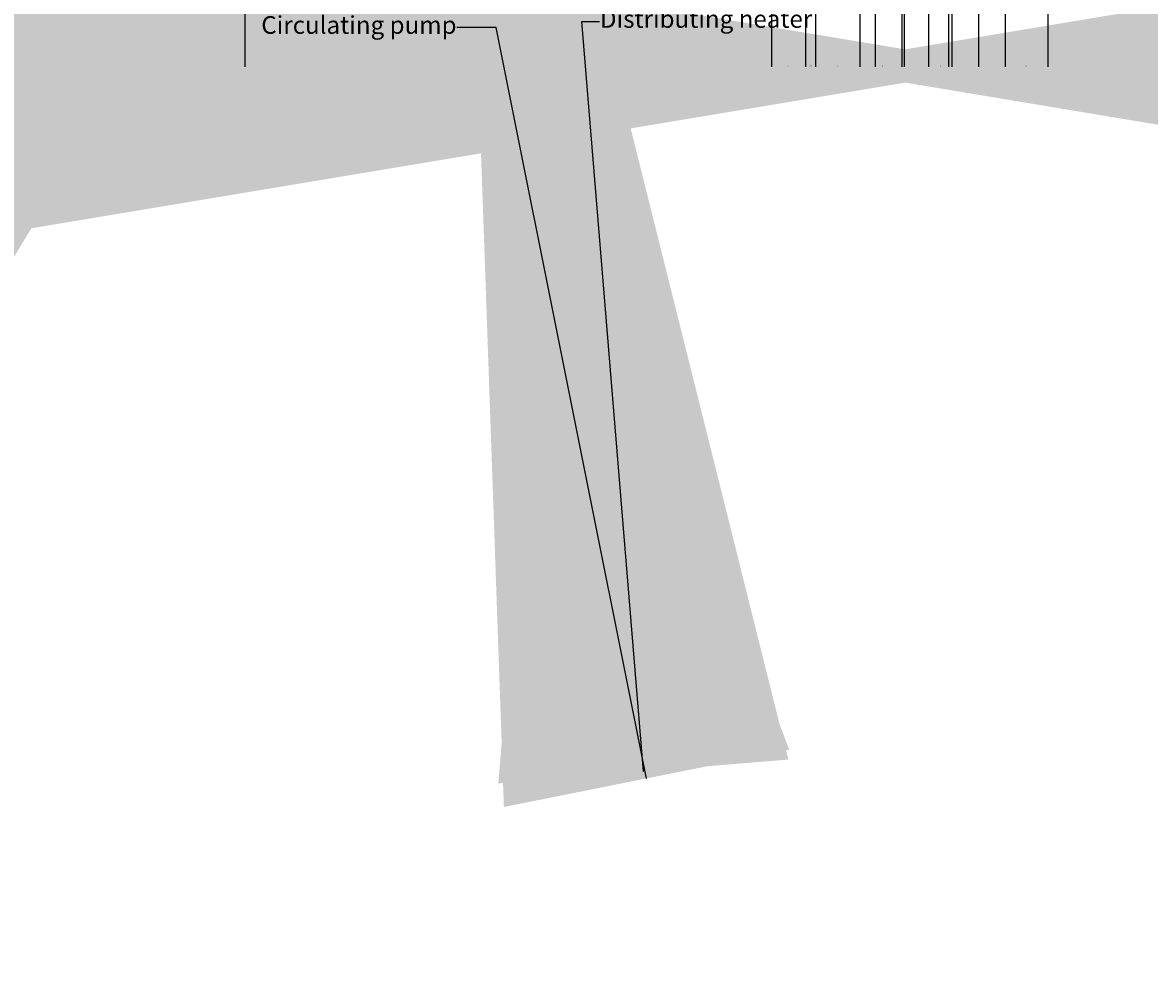
# Model space of a CAD drawing. Units: millimetres. Extents: x -22994 to 29398, y -19990 to 20176.
# Tile 6 of 135: x -44 to 211, y -212 to 5. Entities that reach past the tile are written whole.
import ezdxf
from ezdxf import colors
from ezdxf.entities.mleader import LeaderData, LeaderLine
from ezdxf.math import Vec2, Vec3

# ---------------------------------------------------------------- set-up
doc = ezdxf.new("R2010")
doc.units = ezdxf.units.MM
doc.header["$MEASUREMENT"] = 0
doc.layers.add('M-ANNO-TEXT', color=7, linetype='Continuous', lineweight=25)
doc.layers.add('M-DIMS', color=2, linetype='Continuous', lineweight=18)
doc.styles.get("Standard").update_dxf_attribs({"font": 'arial.ttf'})
doc.dimstyles.get("Standard").update_dxf_attribs({"dimtxt": 0.18, "dimasz": 10000, "dimexe": 0.18, "dimexo": 0.0625, "dimgap": 0.09, "dimtad": 0, "dimtih": 1, "dimtoh": 1, "dimdec": 0, "dimzin": 0, "dimdsep": 46, "dimtxsty": 'Standard', "dimcen": 0.09, "dimadec": 0, "dimazin": 0, "dimtfac": 1, "dimtdec": 0, "dimtofl": 0, "dimtmove": 0, "dimatfit": 3, "dimfxl": 1, "dimtolj": 1, "dimtzin": 0, "dimlwd": 30, "dimarcsym": 0})

# ---------------------------------------------------------------- blocks, each defined once
blk = doc.blocks.new('*D2')
at = {"layer": 'Defpoints', "color": 0, "transparency": 16777216}
for p in [(6.68, 10.27), (290.85, 10.27), (290.85, -5.08)]:
    blk.add_point(p, dxfattribs=at)
at = {"layer": 'M-DIMS', "color": 0, "lineweight": -2, "transparency": 16777216}
for p, q in [((6.68, 10.21), (6.68, -5.26)), ((290.85, 10.21), (290.85, -5.26))]:
    blk.add_line(p, q, dxfattribs=at)
at = {"layer": 'M-DIMS', "color": 0, "lineweight": 30, "transparency": 16777216}
for p, q in [((-9993.32, -5.08), (-19993.32, -5.08)), ((10290.85, -5.08), (20290.85, -5.08))]:
    blk.add_line(p, q, dxfattribs=at)
at = {"layer": 'M-DIMS', "color": 0, "transparency": 16777216}
for points in [[(-9993.32, 1661.59), (-9993.32, -1671.75), (6.68, -5.08)], [(10290.85, 1661.59), (10290.85, -1671.75), (290.85, -5.08)]]:
    blk.add_solid(points, dxfattribs=at)
at = {"layer": 'M-DIMS', "color": 0, "transparency": 16777216, "insert": (148.76, -5.08), "char_height": 0.18, "attachment_point": 5}
blk.add_mtext('\\A1;284.2', dxfattribs=at)
blk = doc.blocks.new('*D3')
at = {"layer": 'Defpoints', "color": 0, "transparency": 16777216}
for p in [(110.26, 204.17), (110.26, 176.37), (95.83, 127.97)]:
    blk.add_point(p, dxfattribs=at)
at = {"layer": 'M-DIMS', "color": 0, "lineweight": 30, "transparency": 16777216}
for p, q in [((-9904.17, 204.17), (-19904.17, 204.17)), ((10110.26, 204.17), (20110.26, 204.17))]:
    blk.add_line(p, q, dxfattribs=at)
at = {"layer": 'M-DIMS', "color": 0, "lineweight": -2, "transparency": 16777216}
for p, q in [((95.83, 128.03), (95.83, 204.35)), ((110.26, 176.43), (110.26, 204.35))]:
    blk.add_line(p, q, dxfattribs=at)
at = {"layer": 'M-DIMS', "color": 0, "transparency": 16777216}
for points in [[(-9904.17, 1870.83), (-9904.17, -1462.5), (95.83, 204.17)], [(10110.26, 1870.83), (10110.26, -1462.5), (110.26, 204.17)]]:
    blk.add_solid(points, dxfattribs=at)
at = {"layer": 'M-DIMS', "color": 0, "transparency": 16777216, "insert": (103.05, 204.17), "char_height": 0.18, "attachment_point": 5}
blk.add_mtext('\\A1;14.432', dxfattribs=at)
blk = doc.blocks.new('*D4')
at = {"layer": 'Defpoints', "color": 0, "transparency": 16777216}
for p in [(116.26, 204.17), (110.26, 176.37), (116.26, 176.37)]:
    blk.add_point(p, dxfattribs=at)
at = {"layer": 'M-DIMS', "color": 0, "lineweight": 30, "transparency": 16777216}
for p, q in [((-9889.74, 204.17), (-19889.74, 204.17)), ((10116.26, 204.17), (20116.26, 204.17))]:
    blk.add_line(p, q, dxfattribs=at)
at = {"layer": 'M-DIMS', "color": 0, "lineweight": -2, "transparency": 16777216}
for p, q in [((110.26, 176.43), (110.26, 204.35)), ((116.26, 176.43), (116.26, 204.35))]:
    blk.add_line(p, q, dxfattribs=at)
at = {"layer": 'M-DIMS', "color": 0, "transparency": 16777216}
for points in [[(-9889.74, 1870.83), (-9889.74, -1462.5), (110.26, 204.17)], [(10116.26, 1870.83), (10116.26, -1462.5), (116.26, 204.17)]]:
    blk.add_solid(points, dxfattribs=at)
at = {"layer": 'M-DIMS', "color": 0, "transparency": 16777216, "insert": (113.26, 204.17), "char_height": 0.18, "attachment_point": 5}
blk.add_mtext('\\A1;6', dxfattribs=at)
blk = doc.blocks.new('*D5')
at = {"layer": 'Defpoints', "color": 0, "transparency": 16777216}
for p in [(181.26, 204.17), (116.26, 176.37), (181.26, 176.37)]:
    blk.add_point(p, dxfattribs=at)
at = {"layer": 'M-DIMS', "color": 0, "lineweight": 30, "transparency": 16777216}
for p, q in [((-9883.74, 204.17), (-19883.74, 204.17)), ((10181.26, 204.17), (20181.26, 204.17))]:
    blk.add_line(p, q, dxfattribs=at)
at = {"layer": 'M-DIMS', "color": 0, "lineweight": -2, "transparency": 16777216}
for p, q in [((116.26, 176.43), (116.26, 204.35)), ((181.26, 176.43), (181.26, 204.35))]:
    blk.add_line(p, q, dxfattribs=at)
at = {"layer": 'M-DIMS', "color": 0, "transparency": 16777216}
for points in [[(-9883.74, 1870.83), (-9883.74, -1462.5), (116.26, 204.17)], [(10181.26, 1870.83), (10181.26, -1462.5), (181.26, 204.17)]]:
    blk.add_solid(points, dxfattribs=at)
at = {"layer": 'M-DIMS', "color": 0, "transparency": 16777216, "insert": (148.76, 204.17), "char_height": 0.18, "attachment_point": 5}
blk.add_mtext('\\A1;65', dxfattribs=at)
blk = doc.blocks.new('*D6')
at = {"layer": 'Defpoints', "color": 0, "transparency": 16777216}
for p in [(187.26, 204.17), (181.26, 176.37), (187.26, 176.37)]:
    blk.add_point(p, dxfattribs=at)
at = {"layer": 'M-DIMS', "color": 0, "lineweight": 30, "transparency": 16777216}
for p, q in [((-9818.74, 204.17), (-19818.74, 204.17)), ((10187.26, 204.17), (20187.26, 204.17))]:
    blk.add_line(p, q, dxfattribs=at)
at = {"layer": 'M-DIMS', "color": 0, "lineweight": -2, "transparency": 16777216}
for p, q in [((181.26, 176.43), (181.26, 204.35)), ((187.26, 176.43), (187.26, 204.35))]:
    blk.add_line(p, q, dxfattribs=at)
at = {"layer": 'M-DIMS', "color": 0, "transparency": 16777216}
for points in [[(-9818.74, 1870.83), (-9818.74, -1462.5), (181.26, 204.17)], [(10187.26, 1870.83), (10187.26, -1462.5), (187.26, 204.17)]]:
    blk.add_solid(points, dxfattribs=at)
at = {"layer": 'M-DIMS', "color": 0, "transparency": 16777216, "insert": (184.26, 204.17), "char_height": 0.18, "attachment_point": 5}
blk.add_mtext('\\A1;6', dxfattribs=at)
blk = doc.blocks.new('*D7')
at = {"layer": 'Defpoints', "color": 0, "transparency": 16777216}
for p in [(201.7, 204.17), (187.26, 176.37), (201.7, 127.97)]:
    blk.add_point(p, dxfattribs=at)
at = {"layer": 'M-DIMS', "color": 0, "lineweight": 30, "transparency": 16777216}
for p, q in [((-9812.74, 204.17), (-19812.74, 204.17)), ((10201.7, 204.17), (20201.7, 204.17))]:
    blk.add_line(p, q, dxfattribs=at)
at = {"layer": 'M-DIMS', "color": 0, "lineweight": -2, "transparency": 16777216}
for p, q in [((187.26, 176.43), (187.26, 204.35)), ((201.7, 128.03), (201.7, 204.35))]:
    blk.add_line(p, q, dxfattribs=at)
at = {"layer": 'M-DIMS', "color": 0, "transparency": 16777216}
for points in [[(-9812.74, 1870.83), (-9812.74, -1462.5), (187.26, 204.17)], [(10201.7, 1870.83), (10201.7, -1462.5), (201.7, 204.17)]]:
    blk.add_solid(points, dxfattribs=at)
at = {"layer": 'M-DIMS', "color": 0, "transparency": 16777216, "insert": (194.48, 204.17), "char_height": 0.18, "attachment_point": 5}
blk.add_mtext('\\A1;14.432', dxfattribs=at)
blk = doc.blocks.new('*D8')
at = {"layer": 'Defpoints', "color": 0, "transparency": 16777216}
for p in [(227.65, 204.17), (227.65, 146.73), (201.7, 127.97)]:
    blk.add_point(p, dxfattribs=at)
at = {"layer": 'M-DIMS', "color": 0, "lineweight": 30, "transparency": 16777216}
for p, q in [((-9798.3, 204.17), (-19798.3, 204.17)), ((10227.65, 204.17), (20227.65, 204.17))]:
    blk.add_line(p, q, dxfattribs=at)
at = {"layer": 'M-DIMS', "color": 0, "lineweight": -2, "transparency": 16777216}
for p, q in [((201.7, 128.03), (201.7, 204.35)), ((227.65, 146.79), (227.65, 204.35))]:
    blk.add_line(p, q, dxfattribs=at)
at = {"layer": 'M-DIMS', "color": 0, "transparency": 16777216}
for points in [[(-9798.3, 1870.83), (-9798.3, -1462.5), (201.7, 204.17)], [(10227.65, 1870.83), (10227.65, -1462.5), (227.65, 204.17)]]:
    blk.add_solid(points, dxfattribs=at)
at = {"layer": 'M-DIMS', "color": 0, "transparency": 16777216, "insert": (214.67, 204.17), "char_height": 0.18, "attachment_point": 5}
blk.add_mtext('\\A1;25.95', dxfattribs=at)
blk = doc.blocks.new('*D9')
at = {"layer": 'Defpoints', "color": 0, "transparency": 16777216}
for p in [(187.26, 176.37), (306.2, 176.37), (290.85, 10.27)]:
    blk.add_point(p, dxfattribs=at)
at = {"layer": 'M-DIMS', "color": 0, "lineweight": 30, "transparency": 16777216}
for p, q in [((306.2, 10176.37), (306.2, 20176.37)), ((306.2, -9989.73), (306.2, -19989.73))]:
    blk.add_line(p, q, dxfattribs=at)
at = {"layer": 'M-DIMS', "color": 0, "lineweight": -2, "transparency": 16777216}
for p, q in [((187.33, 176.37), (306.38, 176.37)), ((290.91, 10.27), (306.38, 10.27))]:
    blk.add_line(p, q, dxfattribs=at)
at = {"layer": 'M-DIMS', "color": 0, "transparency": 16777216}
for points in [[(-1360.46, 10176.37), (1972.87, 10176.37), (306.2, 176.37)], [(-1360.46, -9989.73), (1972.87, -9989.73), (306.2, 10.27)]]:
    blk.add_solid(points, dxfattribs=at)
at = {"layer": 'M-DIMS', "color": 0, "transparency": 16777216, "insert": (306.2, 93.32), "char_height": 0.18, "attachment_point": 5}
blk.add_mtext('\\A1;166.1', dxfattribs=at)
blk = doc.blocks.new('*D10')
at = {"layer": 'Defpoints', "color": 0, "transparency": 16777216}
for p in [(125.65, 136.07), (133.35, 136.07), (133.35, -5.08)]:
    blk.add_point(p, dxfattribs=at)
at = {"layer": 'M-DIMS', "color": 0, "lineweight": -2, "transparency": 16777216}
for p, q in [((125.65, 136.01), (125.65, -5.26)), ((133.35, 136.01), (133.35, -5.26))]:
    blk.add_line(p, q, dxfattribs=at)
at = {"layer": 'M-DIMS', "color": 0, "lineweight": 30, "transparency": 16777216}
for p, q in [((-9874.35, -5.08), (-19874.35, -5.08)), ((10133.35, -5.08), (20133.35, -5.08))]:
    blk.add_line(p, q, dxfattribs=at)
at = {"layer": 'M-DIMS', "color": 0, "transparency": 16777216}
for points in [[(-9874.35, 1661.59), (-9874.35, -1671.75), (125.65, -5.08)], [(10133.35, 1661.59), (10133.35, -1671.75), (133.35, -5.08)]]:
    blk.add_solid(points, dxfattribs=at)
at = {"layer": 'M-DIMS', "color": 0, "transparency": 16777216, "insert": (129.5, -5.08), "char_height": 0.18, "attachment_point": 5}
blk.add_mtext('\\A1;7.696', dxfattribs=at)
blk = doc.blocks.new('*D11')
at = {"layer": 'Defpoints', "color": 0, "transparency": 16777216}
for p in [(133.35, 136.07), (135.65, 136.07), (135.65, -5.08)]:
    blk.add_point(p, dxfattribs=at)
at = {"layer": 'M-DIMS', "color": 0, "lineweight": -2, "transparency": 16777216}
for p, q in [((133.35, 136.01), (133.35, -5.26)), ((135.65, 136.01), (135.65, -5.26))]:
    blk.add_line(p, q, dxfattribs=at)
at = {"layer": 'M-DIMS', "color": 0, "lineweight": 30, "transparency": 16777216}
for p, q in [((-9866.65, -5.08), (-19866.65, -5.08)), ((10135.65, -5.08), (20135.65, -5.08))]:
    blk.add_line(p, q, dxfattribs=at)
at = {"layer": 'M-DIMS', "color": 0, "transparency": 16777216}
for points in [[(-9866.65, 1661.59), (-9866.65, -1671.75), (133.35, -5.08)], [(10135.65, 1661.59), (10135.65, -1671.75), (135.65, -5.08)]]:
    blk.add_solid(points, dxfattribs=at)
at = {"layer": 'M-DIMS', "color": 0, "transparency": 16777216, "insert": (134.5, -5.08), "char_height": 0.18, "attachment_point": 5}
blk.add_mtext('\\A1;2.304', dxfattribs=at)
blk = doc.blocks.new('*D12')
at = {"layer": 'Defpoints', "color": 0, "transparency": 16777216}
for p in [(135.65, 136.07), (145.65, 136.07), (145.65, -5.08)]:
    blk.add_point(p, dxfattribs=at)
at = {"layer": 'M-DIMS', "color": 0, "lineweight": -2, "transparency": 16777216}
for p, q in [((135.65, 136.01), (135.65, -5.26)), ((145.65, 136.01), (145.65, -5.26))]:
    blk.add_line(p, q, dxfattribs=at)
at = {"layer": 'M-DIMS', "color": 0, "lineweight": 30, "transparency": 16777216}
for p, q in [((-9864.35, -5.08), (-19864.35, -5.08)), ((10145.65, -5.08), (20145.65, -5.08))]:
    blk.add_line(p, q, dxfattribs=at)
at = {"layer": 'M-DIMS', "color": 0, "transparency": 16777216}
for points in [[(-9864.35, 1661.59), (-9864.35, -1671.75), (135.65, -5.08)], [(10145.65, 1661.59), (10145.65, -1671.75), (145.65, -5.08)]]:
    blk.add_solid(points, dxfattribs=at)
at = {"layer": 'M-DIMS', "color": 0, "transparency": 16777216, "insert": (140.65, -5.08), "char_height": 0.18, "attachment_point": 5}
blk.add_mtext('\\A1;10', dxfattribs=at)
blk = doc.blocks.new('*D13')
at = {"layer": 'Defpoints', "color": 0, "transparency": 16777216}
for p in [(145.65, 136.07), (155.65, 136.07), (155.65, -5.08)]:
    blk.add_point(p, dxfattribs=at)
at = {"layer": 'M-DIMS', "color": 0, "lineweight": -2, "transparency": 16777216}
for p, q in [((145.65, 136.01), (145.65, -5.26)), ((155.65, 136.01), (155.65, -5.26))]:
    blk.add_line(p, q, dxfattribs=at)
at = {"layer": 'M-DIMS', "color": 0, "lineweight": 30, "transparency": 16777216}
for p, q in [((-9854.35, -5.08), (-19854.35, -5.08)), ((10155.65, -5.08), (20155.65, -5.08))]:
    blk.add_line(p, q, dxfattribs=at)
at = {"layer": 'M-DIMS', "color": 0, "transparency": 16777216}
for points in [[(-9854.35, 1661.59), (-9854.35, -1671.75), (145.65, -5.08)], [(10155.65, 1661.59), (10155.65, -1671.75), (155.65, -5.08)]]:
    blk.add_solid(points, dxfattribs=at)
at = {"layer": 'M-DIMS', "color": 0, "transparency": 16777216, "insert": (150.65, -5.08), "char_height": 0.18, "attachment_point": 5}
blk.add_mtext('\\A1;10', dxfattribs=at)
blk = doc.blocks.new('*D14')
at = {"layer": 'Defpoints', "color": 0, "transparency": 16777216}
for p in [(155.65, 136.07), (165.65, 136.07), (165.65, -5.08)]:
    blk.add_point(p, dxfattribs=at)
at = {"layer": 'M-DIMS', "color": 0, "lineweight": -2, "transparency": 16777216}
for p, q in [((155.65, 136.01), (155.65, -5.26)), ((165.65, 136.01), (165.65, -5.26))]:
    blk.add_line(p, q, dxfattribs=at)
at = {"layer": 'M-DIMS', "color": 0, "lineweight": 30, "transparency": 16777216}
for p, q in [((-9844.35, -5.08), (-19844.35, -5.08)), ((10165.65, -5.08), (20165.65, -5.08))]:
    blk.add_line(p, q, dxfattribs=at)
at = {"layer": 'M-DIMS', "color": 0, "transparency": 16777216}
for points in [[(-9844.35, 1661.59), (-9844.35, -1671.75), (155.65, -5.08)], [(10165.65, 1661.59), (10165.65, -1671.75), (165.65, -5.08)]]:
    blk.add_solid(points, dxfattribs=at)
at = {"layer": 'M-DIMS', "color": 0, "transparency": 16777216, "insert": (160.65, -5.08), "char_height": 0.18, "attachment_point": 5}
blk.add_mtext('\\A1;10', dxfattribs=at)
blk = doc.blocks.new('*D15')
at = {"layer": 'Defpoints', "color": 0, "transparency": 16777216}
for p in [(173.35, 154.79), (173.35, 136.07), (306.2, 136.07)]:
    blk.add_point(p, dxfattribs=at)
at = {"layer": 'M-DIMS', "color": 0, "lineweight": 30, "transparency": 16777216}
for p, q in [((306.2, 10154.79), (306.2, 20154.79)), ((306.2, -9863.93), (306.2, -19863.93))]:
    blk.add_line(p, q, dxfattribs=at)
at = {"layer": 'M-DIMS', "color": 0, "lineweight": -2, "transparency": 16777216}
for p, q in [((173.41, 154.79), (306.38, 154.79)), ((173.41, 136.07), (306.38, 136.07))]:
    blk.add_line(p, q, dxfattribs=at)
at = {"layer": 'M-DIMS', "color": 0, "transparency": 16777216}
for points in [[(-1360.46, 10154.79), (1972.87, 10154.79), (306.2, 154.79)], [(-1360.46, -9863.93), (1972.87, -9863.93), (306.2, 136.07)]]:
    blk.add_solid(points, dxfattribs=at)
at = {"layer": 'M-DIMS', "color": 0, "transparency": 16777216, "insert": (306.2, 145.43), "char_height": 0.18, "attachment_point": 5}
blk.add_mtext('\\A1;18.717', dxfattribs=at)
blk = doc.blocks.new('*D16')
at = {"layer": 'Defpoints', "color": 0, "transparency": 16777216}
for p in [(120.17, 204.17), (110.47, 48.03), (120.17, 48.03)]:
    blk.add_point(p, dxfattribs=at)
at = {"layer": 'M-DIMS', "color": 0, "lineweight": 30, "transparency": 16777216}
for p, q in [((-9889.53, 204.17), (-19889.53, 204.17)), ((10120.17, 204.17), (20120.17, 204.17))]:
    blk.add_line(p, q, dxfattribs=at)
at = {"layer": 'M-DIMS', "color": 0, "lineweight": -2, "transparency": 16777216}
for p, q in [((110.47, 48.1), (110.47, 204.35)), ((120.17, 48.1), (120.17, 204.35))]:
    blk.add_line(p, q, dxfattribs=at)
at = {"layer": 'M-DIMS', "color": 0, "transparency": 16777216}
for points in [[(-9889.53, 1870.83), (-9889.53, -1462.5), (110.47, 204.17)], [(10120.17, 1870.83), (10120.17, -1462.5), (120.17, 204.17)]]:
    blk.add_solid(points, dxfattribs=at)
at = {"layer": 'M-DIMS', "color": 0, "transparency": 16777216, "insert": (115.32, 204.17), "char_height": 0.18, "attachment_point": 5}
blk.add_mtext('\\A1;9.704', dxfattribs=at)
blk = doc.blocks.new('*D17')
at = {"layer": 'Defpoints', "color": 0, "transparency": 16777216}
for p in [(126.17, 204.17), (120.17, 48.03), (126.17, 48.03)]:
    blk.add_point(p, dxfattribs=at)
at = {"layer": 'M-DIMS', "color": 0, "lineweight": 30, "transparency": 16777216}
for p, q in [((-9879.83, 204.17), (-19879.83, 204.17)), ((10126.17, 204.17), (20126.17, 204.17))]:
    blk.add_line(p, q, dxfattribs=at)
at = {"layer": 'M-DIMS', "color": 0, "lineweight": -2, "transparency": 16777216}
for p, q in [((120.17, 48.1), (120.17, 204.35)), ((126.17, 48.1), (126.17, 204.35))]:
    blk.add_line(p, q, dxfattribs=at)
at = {"layer": 'M-DIMS', "color": 0, "transparency": 16777216}
for points in [[(-9879.83, 1870.83), (-9879.83, -1462.5), (120.17, 204.17)], [(10126.17, 1870.83), (10126.17, -1462.5), (126.17, 204.17)]]:
    blk.add_solid(points, dxfattribs=at)
at = {"layer": 'M-DIMS', "color": 0, "transparency": 16777216, "insert": (123.17, 204.17), "char_height": 0.18, "attachment_point": 5}
blk.add_mtext('\\A1;6', dxfattribs=at)
blk = doc.blocks.new('*D18')
at = {"layer": 'Defpoints', "color": 0, "transparency": 16777216}
for p in [(132.17, 204.17), (126.17, 48.03), (132.17, 48.03)]:
    blk.add_point(p, dxfattribs=at)
at = {"layer": 'M-DIMS', "color": 0, "lineweight": 30, "transparency": 16777216}
for p, q in [((-9873.83, 204.17), (-19873.83, 204.17)), ((10132.17, 204.17), (20132.17, 204.17))]:
    blk.add_line(p, q, dxfattribs=at)
at = {"layer": 'M-DIMS', "color": 0, "lineweight": -2, "transparency": 16777216}
for p, q in [((126.17, 48.1), (126.17, 204.35)), ((132.17, 48.1), (132.17, 204.35))]:
    blk.add_line(p, q, dxfattribs=at)
at = {"layer": 'M-DIMS', "color": 0, "transparency": 16777216}
for points in [[(-9873.83, 1870.83), (-9873.83, -1462.5), (126.17, 204.17)], [(10132.17, 1870.83), (10132.17, -1462.5), (132.17, 204.17)]]:
    blk.add_solid(points, dxfattribs=at)
at = {"layer": 'M-DIMS', "color": 0, "transparency": 16777216, "insert": (129.17, 204.17), "char_height": 0.18, "attachment_point": 5}
blk.add_mtext('\\A1;6', dxfattribs=at)
blk = doc.blocks.new('*D19')
at = {"layer": 'Defpoints', "color": 0, "transparency": 16777216}
for p in [(138.17, 204.17), (132.17, 48.03), (138.17, 48.03)]:
    blk.add_point(p, dxfattribs=at)
at = {"layer": 'M-DIMS', "color": 0, "lineweight": 30, "transparency": 16777216}
for p, q in [((-9867.83, 204.17), (-19867.83, 204.17)), ((10138.17, 204.17), (20138.17, 204.17))]:
    blk.add_line(p, q, dxfattribs=at)
at = {"layer": 'M-DIMS', "color": 0, "lineweight": -2, "transparency": 16777216}
for p, q in [((132.17, 48.1), (132.17, 204.35)), ((138.17, 48.1), (138.17, 204.35))]:
    blk.add_line(p, q, dxfattribs=at)
at = {"layer": 'M-DIMS', "color": 0, "transparency": 16777216}
for points in [[(-9867.83, 1870.83), (-9867.83, -1462.5), (132.17, 204.17)], [(10138.17, 1870.83), (10138.17, -1462.5), (138.17, 204.17)]]:
    blk.add_solid(points, dxfattribs=at)
at = {"layer": 'M-DIMS', "color": 0, "transparency": 16777216, "insert": (135.17, 204.17), "char_height": 0.18, "attachment_point": 5}
blk.add_mtext('\\A1;6', dxfattribs=at)
blk = doc.blocks.new('*D20')
at = {"layer": 'Defpoints', "color": 0, "transparency": 16777216}
for p in [(144.17, 204.17), (138.17, 48.03), (144.17, 48.03)]:
    blk.add_point(p, dxfattribs=at)
at = {"layer": 'M-DIMS', "color": 0, "lineweight": 30, "transparency": 16777216}
for p, q in [((-9861.83, 204.17), (-19861.83, 204.17)), ((10144.17, 204.17), (20144.17, 204.17))]:
    blk.add_line(p, q, dxfattribs=at)
at = {"layer": 'M-DIMS', "color": 0, "lineweight": -2, "transparency": 16777216}
for p, q in [((138.17, 48.1), (138.17, 204.35)), ((144.17, 48.1), (144.17, 204.35))]:
    blk.add_line(p, q, dxfattribs=at)
at = {"layer": 'M-DIMS', "color": 0, "transparency": 16777216}
for points in [[(-9861.83, 1870.83), (-9861.83, -1462.5), (138.17, 204.17)], [(10144.17, 1870.83), (10144.17, -1462.5), (144.17, 204.17)]]:
    blk.add_solid(points, dxfattribs=at)
at = {"layer": 'M-DIMS', "color": 0, "transparency": 16777216, "insert": (141.17, 204.17), "char_height": 0.18, "attachment_point": 5}
blk.add_mtext('\\A1;6', dxfattribs=at)
blk = doc.blocks.new('*D21')
at = {"layer": 'Defpoints', "color": 0, "transparency": 16777216}
for p in [(149.12, 204.17), (144.17, 48.03), (149.12, 48.03)]:
    blk.add_point(p, dxfattribs=at)
at = {"layer": 'M-DIMS', "color": 0, "lineweight": 30, "transparency": 16777216}
for p, q in [((-9855.83, 204.17), (-19855.83, 204.17)), ((10149.12, 204.17), (20149.12, 204.17))]:
    blk.add_line(p, q, dxfattribs=at)
at = {"layer": 'M-DIMS', "color": 0, "lineweight": -2, "transparency": 16777216}
for p, q in [((144.17, 48.1), (144.17, 204.35)), ((149.12, 48.1), (149.12, 204.35))]:
    blk.add_line(p, q, dxfattribs=at)
at = {"layer": 'M-DIMS', "color": 0, "transparency": 16777216}
for points in [[(-9855.83, 1870.83), (-9855.83, -1462.5), (144.17, 204.17)], [(10149.12, 1870.83), (10149.12, -1462.5), (149.12, 204.17)]]:
    blk.add_solid(points, dxfattribs=at)
at = {"layer": 'M-DIMS', "color": 0, "transparency": 16777216, "insert": (146.64, 204.17), "char_height": 0.18, "attachment_point": 5}
blk.add_mtext('\\A1;4.945', dxfattribs=at)
blk = doc.blocks.new('*D22')
at = {"layer": 'Defpoints', "color": 0, "transparency": 16777216}
for p in [(149.12, 30.99), (155.12, 30.99), (155.12, -5.08)]:
    blk.add_point(p, dxfattribs=at)
at = {"layer": 'M-DIMS', "color": 0, "lineweight": -2, "transparency": 16777216}
for p, q in [((149.12, 30.93), (149.12, -5.26)), ((155.12, 30.93), (155.12, -5.26))]:
    blk.add_line(p, q, dxfattribs=at)
at = {"layer": 'M-DIMS', "color": 0, "lineweight": 30, "transparency": 16777216}
for p, q in [((-9850.88, -5.08), (-19850.88, -5.08)), ((10155.12, -5.08), (20155.12, -5.08))]:
    blk.add_line(p, q, dxfattribs=at)
at = {"layer": 'M-DIMS', "color": 0, "transparency": 16777216}
for points in [[(-9850.88, 1661.59), (-9850.88, -1671.75), (149.12, -5.08)], [(10155.12, 1661.59), (10155.12, -1671.75), (155.12, -5.08)]]:
    blk.add_solid(points, dxfattribs=at)
at = {"layer": 'M-DIMS', "color": 0, "transparency": 16777216, "insert": (152.12, -5.08), "char_height": 0.18, "attachment_point": 5}
blk.add_mtext('\\A1;6', dxfattribs=at)
blk = doc.blocks.new('*D23')
at = {"layer": 'Defpoints', "color": 0, "transparency": 16777216}
for p in [(155.12, 30.99), (161.12, 30.99), (161.12, -5.08)]:
    blk.add_point(p, dxfattribs=at)
at = {"layer": 'M-DIMS', "color": 0, "lineweight": -2, "transparency": 16777216}
for p, q in [((155.12, 30.93), (155.12, -5.26)), ((161.12, 30.93), (161.12, -5.26))]:
    blk.add_line(p, q, dxfattribs=at)
at = {"layer": 'M-DIMS', "color": 0, "lineweight": 30, "transparency": 16777216}
for p, q in [((-9844.88, -5.08), (-19844.88, -5.08)), ((10161.12, -5.08), (20161.12, -5.08))]:
    blk.add_line(p, q, dxfattribs=at)
at = {"layer": 'M-DIMS', "color": 0, "transparency": 16777216}
for points in [[(-9844.88, 1661.59), (-9844.88, -1671.75), (155.12, -5.08)], [(10161.12, 1661.59), (10161.12, -1671.75), (161.12, -5.08)]]:
    blk.add_solid(points, dxfattribs=at)
at = {"layer": 'M-DIMS', "color": 0, "transparency": 16777216, "insert": (158.12, -5.08), "char_height": 0.18, "attachment_point": 5}
blk.add_mtext('\\A1;6', dxfattribs=at)
blk = doc.blocks.new('*D24')
at = {"layer": 'Defpoints', "color": 0, "transparency": 16777216}
for p in [(161.12, 30.99), (166.44, 30.99), (166.44, -5.08)]:
    blk.add_point(p, dxfattribs=at)
at = {"layer": 'M-DIMS', "color": 0, "lineweight": -2, "transparency": 16777216}
for p, q in [((161.12, 30.93), (161.12, -5.26)), ((166.44, 30.93), (166.44, -5.26))]:
    blk.add_line(p, q, dxfattribs=at)
at = {"layer": 'M-DIMS', "color": 0, "lineweight": 30, "transparency": 16777216}
for p, q in [((-9838.88, -5.08), (-19838.88, -5.08)), ((10166.44, -5.08), (20166.44, -5.08))]:
    blk.add_line(p, q, dxfattribs=at)
at = {"layer": 'M-DIMS', "color": 0, "transparency": 16777216}
for points in [[(-9838.88, 1661.59), (-9838.88, -1671.75), (161.12, -5.08)], [(10166.44, 1661.59), (10166.44, -1671.75), (166.44, -5.08)]]:
    blk.add_solid(points, dxfattribs=at)
at = {"layer": 'M-DIMS', "color": 0, "transparency": 16777216, "insert": (163.78, -5.08), "char_height": 0.18, "attachment_point": 5}
blk.add_mtext('\\A1;5.323', dxfattribs=at)
blk = doc.blocks.new('*D25')
at = {"layer": 'Defpoints', "color": 0, "transparency": 16777216}
for p in [(166.44, 30.99), (172.44, 30.99), (172.44, -5.08)]:
    blk.add_point(p, dxfattribs=at)
at = {"layer": 'M-DIMS', "color": 0, "lineweight": -2, "transparency": 16777216}
for p, q in [((166.44, 30.93), (166.44, -5.26)), ((172.44, 30.93), (172.44, -5.26))]:
    blk.add_line(p, q, dxfattribs=at)
at = {"layer": 'M-DIMS', "color": 0, "lineweight": 30, "transparency": 16777216}
for p, q in [((-9833.56, -5.08), (-19833.56, -5.08)), ((10172.44, -5.08), (20172.44, -5.08))]:
    blk.add_line(p, q, dxfattribs=at)
at = {"layer": 'M-DIMS', "color": 0, "transparency": 16777216}
for points in [[(-9833.56, 1661.59), (-9833.56, -1671.75), (166.44, -5.08)], [(10172.44, 1661.59), (10172.44, -1671.75), (172.44, -5.08)]]:
    blk.add_solid(points, dxfattribs=at)
at = {"layer": 'M-DIMS', "color": 0, "transparency": 16777216, "insert": (169.44, -5.08), "char_height": 0.18, "attachment_point": 5}
blk.add_mtext('\\A1;6', dxfattribs=at)
blk = doc.blocks.new('*D26')
at = {"layer": 'Defpoints', "color": 0, "transparency": 16777216}
for p in [(172.44, 30.99), (178.44, 30.99), (178.44, -5.08)]:
    blk.add_point(p, dxfattribs=at)
at = {"layer": 'M-DIMS', "color": 0, "lineweight": -2, "transparency": 16777216}
for p, q in [((172.44, 30.93), (172.44, -5.26)), ((178.44, 30.93), (178.44, -5.26))]:
    blk.add_line(p, q, dxfattribs=at)
at = {"layer": 'M-DIMS', "color": 0, "lineweight": 30, "transparency": 16777216}
for p, q in [((-9827.56, -5.08), (-19827.56, -5.08)), ((10178.44, -5.08), (20178.44, -5.08))]:
    blk.add_line(p, q, dxfattribs=at)
at = {"layer": 'M-DIMS', "color": 0, "transparency": 16777216}
for points in [[(-9827.56, 1661.59), (-9827.56, -1671.75), (172.44, -5.08)], [(10178.44, 1661.59), (10178.44, -1671.75), (178.44, -5.08)]]:
    blk.add_solid(points, dxfattribs=at)
at = {"layer": 'M-DIMS', "color": 0, "transparency": 16777216, "insert": (175.44, -5.08), "char_height": 0.18, "attachment_point": 5}
blk.add_mtext('\\A1;6', dxfattribs=at)
blk = doc.blocks.new('*D27')
at = {"layer": 'Defpoints', "color": 0, "transparency": 16777216}
for p in [(178.44, 30.99), (188.12, 30.99), (188.12, -5.08)]:
    blk.add_point(p, dxfattribs=at)
at = {"layer": 'M-DIMS', "color": 0, "lineweight": -2, "transparency": 16777216}
for p, q in [((178.44, 30.93), (178.44, -5.26)), ((188.12, 30.93), (188.12, -5.26))]:
    blk.add_line(p, q, dxfattribs=at)
at = {"layer": 'M-DIMS', "color": 0, "lineweight": 30, "transparency": 16777216}
for p, q in [((-9821.56, -5.08), (-19821.56, -5.08)), ((10188.12, -5.08), (20188.12, -5.08))]:
    blk.add_line(p, q, dxfattribs=at)
at = {"layer": 'M-DIMS', "color": 0, "transparency": 16777216}
for points in [[(-9821.56, 1661.59), (-9821.56, -1671.75), (178.44, -5.08)], [(10188.12, 1661.59), (10188.12, -1671.75), (188.12, -5.08)]]:
    blk.add_solid(points, dxfattribs=at)
at = {"layer": 'M-DIMS', "color": 0, "transparency": 16777216, "insert": (183.28, -5.08), "char_height": 0.18, "attachment_point": 5}
blk.add_mtext('\\A1;9.679', dxfattribs=at)
blk = doc.blocks.new('*D28')
at = {"layer": 'Defpoints', "color": 0, "transparency": 16777216}
for p in [(188.12, 48.03), (306.2, 48.03), (188.12, 30.99)]:
    blk.add_point(p, dxfattribs=at)
at = {"layer": 'M-DIMS', "color": 0, "lineweight": 30, "transparency": 16777216}
for p, q in [((306.2, 10048.03), (306.2, 20048.03)), ((306.2, -9969.01), (306.2, -19969.01))]:
    blk.add_line(p, q, dxfattribs=at)
at = {"layer": 'M-DIMS', "color": 0, "lineweight": -2, "transparency": 16777216}
for p, q in [((188.18, 48.03), (306.38, 48.03)), ((188.18, 30.99), (306.38, 30.99))]:
    blk.add_line(p, q, dxfattribs=at)
at = {"layer": 'M-DIMS', "color": 0, "transparency": 16777216}
for points in [[(-1360.46, 10048.03), (1972.87, 10048.03), (306.2, 48.03)], [(-1360.46, -9969.01), (1972.87, -9969.01), (306.2, 30.99)]]:
    blk.add_solid(points, dxfattribs=at)
at = {"layer": 'M-DIMS', "color": 0, "transparency": 16777216, "insert": (306.2, 39.51), "char_height": 0.18, "attachment_point": 5}
blk.add_mtext('\\A1;17.045', dxfattribs=at)
blk = doc.blocks.new('*D29')
at = {"layer": 'Defpoints', "color": 0, "transparency": 16777216}
for p in [(36.8, 80.04), (64.03, 80.04)]:
    blk.add_point(p, dxfattribs=at)
at = {"layer": 'M-DIMS', "color": 0, "lineweight": -2, "transparency": 16777216}
for p, q in [((50.33, 80.04), (50.51, 80.04)), ((50.42, 79.96), (50.42, 80.14))]:
    blk.add_line(p, q, dxfattribs=at)
at = {"layer": 'M-DIMS', "color": 0, "lineweight": 30, "transparency": 16777216}
blk.add_line((20064.03, 80.03), (10064.03, 80.04), dxfattribs=at)
at = {"layer": 'M-DIMS', "color": 0, "transparency": 16777216}
blk.add_solid([(10064.03, 1746.7), (10064.03, -1586.63), (64.03, 80.04)], dxfattribs=at)
at = {"layer": 'M-DIMS', "color": 0, "transparency": 16777216, "insert": (20064.52, 80.03), "char_height": 0.18, "attachment_point": 5}
blk.add_mtext('\\A1;∅27.23', dxfattribs=at)
blk = doc.blocks.new('*D32')
at = {"layer": 'Defpoints', "color": 0, "transparency": 16777216}
for p in [(57.16, 118.61), (52.41, 113.09)]:
    blk.add_point(p, dxfattribs=at)
at = {"layer": 'M-DIMS', "color": 0, "lineweight": -2, "transparency": 16777216}
for p, q in [((57.07, 118.61), (57.25, 118.61)), ((57.16, 118.52), (57.16, 118.7))]:
    blk.add_line(p, q, dxfattribs=at)
at = {"layer": 'M-DIMS', "color": 0, "lineweight": 30, "transparency": 16777216}
for p, q in [((-12992.53, -15047.03), (-6470.06, -7466.97)), ((-22992.53, -15047.03), (-12992.53, -15047.03))]:
    blk.add_line(p, q, dxfattribs=at)
at = {"layer": 'M-DIMS', "color": 0, "transparency": 16777216}
blk.add_solid([(-7733.4, -6379.89), (-5206.72, -8554.05), (52.41, 113.09)], dxfattribs=at)
at = {"layer": 'M-DIMS', "color": 0, "transparency": 16777216, "insert": (-22993.21, -15047.03), "char_height": 0.18, "attachment_point": 5}
blk.add_mtext('\\A1;2X R7.284', dxfattribs=at)
blk = doc.blocks.new('*D37')
at = {"layer": 'Defpoints', "color": 0, "transparency": 16777216}
for p in [(54.83, 118.61), (59.49, 118.61)]:
    blk.add_point(p, dxfattribs=at)
at = {"layer": 'M-DIMS', "color": 0, "lineweight": -2, "transparency": 16777216}
for p, q in [((57.07, 118.61), (57.25, 118.61)), ((57.16, 118.52), (57.16, 118.7))]:
    blk.add_line(p, q, dxfattribs=at)
at = {"layer": 'M-DIMS', "color": 0, "lineweight": 30, "transparency": 16777216}
blk.add_line((20059.49, 116.25), (10059.49, 117.43), dxfattribs=at)
at = {"layer": 'M-DIMS', "color": 0, "transparency": 16777216}
blk.add_solid([(10059.69, 1784.1), (10059.3, -1549.23), (59.49, 118.61)], dxfattribs=at)
at = {"layer": 'M-DIMS', "color": 0, "transparency": 16777216, "insert": (20059.99, 116.25), "char_height": 0.18, "attachment_point": 5}
blk.add_mtext('\\A1;∅4.659', dxfattribs=at)

msp = doc.modelspace()

# ---------------------------------------------------------------- dimensions: what is measured, and where the dimension line sits
at = {"layer": 'M-DIMS'}
for base, p1, p2, override, picture, middle in [((306.202, 176.3662), (290.852, 10.2713), (187.2647, 176.3662), {"dimdec": 1, "dimlfac": 1, "dimrnd": 0, "dimzin": 0, "dimdsep": 46, "dimlunit": 2}, '*D9', (306.202, 93.3187)), ((306.202, 136.0713), (173.3459, 154.788), (173.3459, 136.0713), {"dimdec": 3, "dimlfac": 1, "dimrnd": 0, "dimzin": 0, "dimdsep": 46, "dimlunit": 2}, '*D15', (306.202, 145.4297)), ((306.202, 48.0349), (188.1175, 30.9895), (188.1175, 48.0349), {"dimdec": 3, "dimlfac": 1, "dimrnd": 0, "dimzin": 0, "dimdsep": 46, "dimlunit": 2}, '*D28', (306.202, 39.5122))]:
    dim = msp.add_linear_dim(base=base, p1=p1, p2=p2, angle=90, dimstyle='Standard', override=override, dxfattribs=at)
    dim.commit()
    dim.dimension.update_dxf_attribs({"geometry": picture, "text_midpoint": middle})
for base, p1, p2, override, picture, middle in [((110.2647, 204.1654), (95.8327, 127.967), (110.2647, 176.3662), {"dimdec": 3, "dimlfac": 1, "dimrnd": 0, "dimzin": 0, "dimdsep": 46, "dimlunit": 2}, '*D3', (103.0487, 204.1654)), ((116.2647, 204.1654), (110.2647, 176.3662), (116.2647, 176.3662), {"dimdec": 0, "dimlfac": 1, "dimrnd": 0, "dimzin": 0, "dimdsep": 46, "dimlunit": 2}, '*D4', (113.2647, 204.1654)), ((120.1702, 204.1654), (110.4658, 48.0349), (120.1702, 48.0349), {"dimdec": 3, "dimlfac": 1, "dimrnd": 0, "dimzin": 0, "dimdsep": 46, "dimlunit": 2}, '*D16', (115.318, 204.1654)), ((181.2647, 204.1654), (116.2647, 176.3662), (181.2647, 176.3662), {"dimdec": 0, "dimlfac": 1, "dimrnd": 0, "dimzin": 0, "dimdsep": 46, "dimlunit": 2}, '*D5', (148.7647, 204.1654)), ((126.1702, 204.1654), (120.1702, 48.0349), (126.1702, 48.0349), {"dimdec": 0, "dimlfac": 1, "dimrnd": 0, "dimzin": 0, "dimdsep": 46, "dimlunit": 2}, '*D17', (123.1702, 204.1654)), ((132.1702, 204.1654), (126.1702, 48.0349), (132.1702, 48.0349), {"dimdec": 0, "dimlfac": 1, "dimrnd": 0, "dimzin": 0, "dimdsep": 46, "dimlunit": 2}, '*D18', (129.1702, 204.1654)), ((138.1702, 204.1654), (132.1702, 48.0349), (138.1702, 48.0349), {"dimdec": 0, "dimlfac": 1, "dimrnd": 0, "dimzin": 0, "dimdsep": 46, "dimlunit": 2}, '*D19', (135.1702, 204.1654)), ((144.1702, 204.1654), (138.1702, 48.0349), (144.1702, 48.0349), {"dimdec": 0, "dimlfac": 1, "dimrnd": 0, "dimzin": 0, "dimdsep": 46, "dimlunit": 2}, '*D20', (141.1702, 204.1654)), ((149.11567, 204.16539), (144.17023, 48.03494), (149.11567, 48.03494), {"dimdec": 3, "dimlfac": 1, "dimrnd": 0, "dimzin": 0, "dimdsep": 46, "dimlunit": 2}, '*D21', (146.64295, 204.16539)), ((187.2647, 204.1654), (181.2647, 176.3662), (187.2647, 176.3662), {"dimdec": 0, "dimlfac": 1, "dimrnd": 0, "dimzin": 0, "dimdsep": 46, "dimlunit": 2}, '*D6', (184.2647, 204.1654)), ((201.6967, 204.1654), (187.2647, 176.3662), (201.6967, 127.967), {"dimdec": 3, "dimlfac": 1, "dimrnd": 0, "dimzin": 0, "dimdsep": 46, "dimlunit": 2}, '*D7', (194.4807, 204.1654)), ((227.6485, 204.1654), (201.6967, 127.967), (227.6485, 146.7296), {"dimdec": 2, "dimlfac": 1, "dimrnd": 0, "dimzin": 0, "dimdsep": 46, "dimlunit": 2}, '*D8', (214.6726, 204.1654)), ((290.852, -5.0787), (6.6773, 10.2713), (290.852, 10.2713), {"dimdec": 1, "dimlfac": 1, "dimrnd": 0, "dimzin": 0, "dimdsep": 46, "dimlunit": 2}, '*D2', (148.7647, -5.0787)), ((133.3459, -5.0787), (125.6498, 136.0713), (133.3459, 136.0713), {"dimdec": 3, "dimlfac": 1, "dimrnd": 0, "dimzin": 0, "dimdsep": 46, "dimlunit": 2}, '*D10', (129.4978, -5.0787)), ((135.6498, -5.0787), (133.3459, 136.0713), (135.6498, 136.0713), {"dimdec": 3, "dimlfac": 1, "dimrnd": 0, "dimzin": 0, "dimdsep": 46, "dimlunit": 2}, '*D11', (134.4978, -5.0787)), ((145.6498, -5.0787), (135.6498, 136.0713), (145.6498, 136.0713), {"dimdec": 0, "dimlfac": 1, "dimrnd": 0, "dimzin": 0, "dimdsep": 46, "dimlunit": 2}, '*D12', (140.6498, -5.0787)), ((155.6498, -5.0787), (145.6498, 136.0713), (155.6498, 136.0713), {"dimdec": 0, "dimlfac": 1, "dimrnd": 0, "dimzin": 0, "dimdsep": 46, "dimlunit": 2}, '*D13', (150.6498, -5.0787)), ((155.1157, -5.0787), (149.1157, 30.9895), (155.1157, 30.9895), {"dimdec": 0, "dimlfac": 1, "dimrnd": 0, "dimzin": 0, "dimdsep": 46, "dimlunit": 2}, '*D22', (152.1157, -5.0787)), ((161.1157, -5.0787), (155.1157, 30.9895), (161.1157, 30.9895), {"dimdec": 0, "dimlfac": 1, "dimrnd": 0, "dimzin": 0, "dimdsep": 46, "dimlunit": 2}, '*D23', (158.1157, -5.0787)), ((165.6498, -5.0787), (155.6498, 136.0713), (165.6498, 136.0713), {"dimdec": 0, "dimlfac": 1, "dimrnd": 0, "dimzin": 0, "dimdsep": 46, "dimlunit": 2}, '*D14', (160.6498, -5.0787)), ((166.4387, -5.0787), (161.1157, 30.9895), (166.4387, 30.9895), {"dimdec": 3, "dimlfac": 1, "dimrnd": 0, "dimzin": 0, "dimdsep": 46, "dimlunit": 2}, '*D24', (163.7772, -5.0787)), ((172.4387, -5.0787), (166.4387, 30.9895), (172.4387, 30.9895), {"dimdec": 0, "dimlfac": 1, "dimrnd": 0, "dimzin": 0, "dimdsep": 46, "dimlunit": 2}, '*D25', (169.4387, -5.0787)), ((178.4387, -5.0787), (172.4387, 30.9895), (178.4387, 30.9895), {"dimdec": 0, "dimlfac": 1, "dimrnd": 0, "dimzin": 0, "dimdsep": 46, "dimlunit": 2}, '*D26', (175.4387, -5.0787)), ((188.1175, -5.0787), (178.4387, 30.9895), (188.1175, 30.9895), {"dimdec": 3, "dimlfac": 1, "dimrnd": 0, "dimzin": 0, "dimdsep": 46, "dimlunit": 2}, '*D27', (183.2781, -5.0787))]:
    dim = msp.add_linear_dim(base=base, p1=p1, p2=p2, dimstyle='Standard', override=override, dxfattribs=at)
    dim.commit()
    dim.dimension.update_dxf_attribs({"geometry": picture, "text_midpoint": middle})
for p1, p2, override, picture, middle in [((54.8343, 118.6145), (59.4936, 118.614), {"dimdec": 3, "dimlfac": 1, "dimrnd": 0, "dimzin": 0, "dimdsep": 46, "dimlunit": 2}, '*D37', (20059.4934, 116.2531)), ((36.8006, 80.045), (64.0296, 80.045), {"dimdec": 2, "dimlfac": 1, "dimrnd": 0, "dimzin": 0, "dimdsep": 46, "dimlunit": 2}, '*D29', (20064.0296, 80.0303))]:
    dim = msp.add_diameter_dim_2p(p1=p1, p2=p2, dimstyle='Standard', override=override, dxfattribs=at)
    dim.commit()
    dim.dimension.update_dxf_attribs({"geometry": picture, "text_midpoint": middle})
dim = msp.add_radius_dim(center=(57.1639, 118.6143), mpoint=(52.4129, 113.0929), text='2X <>', dimstyle='Standard', override={"dimdec": 3, "dimlfac": 1, "dimrnd": 0, "dimzin": 0, "dimdsep": 46, "dimlunit": 2}, dxfattribs=at)
dim.commit()
dim.dimension.update_dxf_attribs({"geometry": '*D32', "text_midpoint": (-22993.208, -15047.0314)})

# ---------------------------------------------------------------- leaders
at = {"layer": 'M-ANNO-TEXT'}
ml = msp.add_multileader_mtext('Standard', dxfattribs=at)
ml.set_content('Distributing heater', color=256)
ml.set_leader_properties()
ml.build(insert=Vec2(0, 0))
ml.multileader.update_dxf_attribs({"dogleg_length": 0.36, "arrow_head_size": 200})
ctx = ml.context
ctx.base_point, ctx.arrow_head_size, ctx.landing_gap_size, ctx.plane_origin = Vec3(86.8201, 4.9577), 200, 0.09, Vec3(80.3507, 34.8308)
notes = []
notes.append((ctx, [(1, (1, 1, 0), (82.8058, 4.9577), (1, 0), 4.0143, [(0, [(80.3507, 34.8308)], 0, [])])]))
ctx.mtext.insert, ctx.mtext.flow_direction = Vec3(86.9101, 7.5457), 5
ml = msp.add_multileader_mtext('Standard', dxfattribs=at)
ml.set_content('Circulating pump', color=256)
ml.set_leader_properties()
ml.build(insert=Vec2(0, 0))
ml.multileader.update_dxf_attribs({"dogleg_length": 0.36, "arrow_head_size": 200})
ctx = ml.context
ctx.base_point, ctx.arrow_head_size, ctx.landing_gap_size, ctx.plane_origin = Vec3(13.008, 3.5951), 200, 0.09, Vec3(56.3887, 19.3615)
ctx.text_align_type = 2
notes.append((ctx, [(1, (1, 1, 0), (63.4296, 3.5951), (-1, 0), 8.8146, [(0, [(58.1278, 30.0354)], 0, [])])]))
ctx.mtext.insert, ctx.mtext.alignment, ctx.mtext.flow_direction = Vec3(54.525, 6.1831), 3, 5
for ctx, leaders in notes:
    for number, flags, end, landing, length, lines in leaders:
        leader = LeaderData()
        leader.index, (leader.has_last_leader_line, leader.has_dogleg_vector, leader.attachment_direction) = number, flags
        leader.last_leader_point, leader.dogleg_vector, leader.dogleg_length = Vec3(end), Vec3(landing), length
        for number, points, colour, breaks in lines:
            line = LeaderLine()
            line.index, line.vertices, line.color, line.breaks = number, Vec3.list(points), colors.encode_raw_color(colour), breaks
            leader.lines.append(line)
        ctx.leaders.append(leader)

doc.saveas('drawing.dxf')
